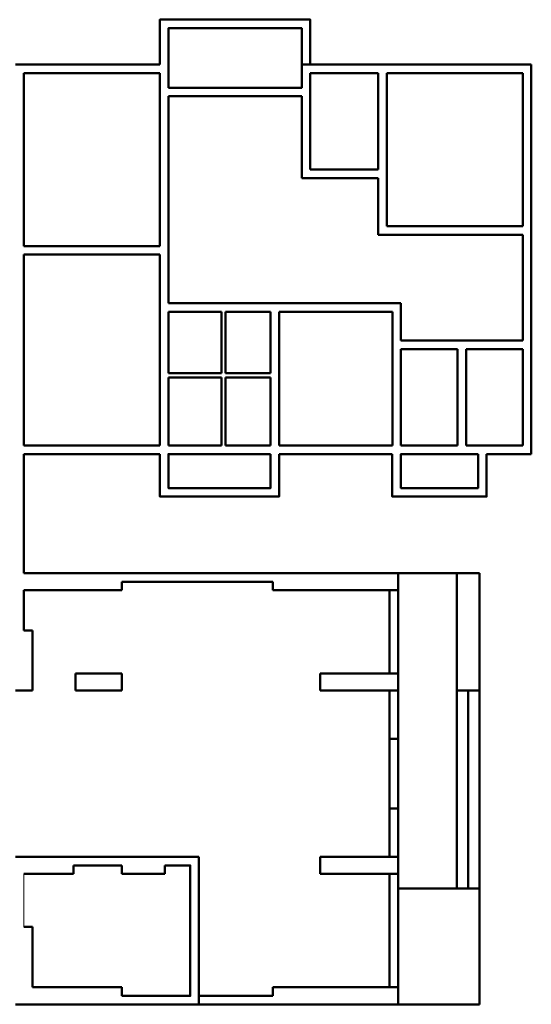
# Model space of a CAD drawing. Units: inches. Extents: x -105 to 1531, y -656 to 2003.
# Tile 6 of 6: x 979 to 1521, y 44 to 1085. Entities that reach past the tile are written whole.
import ezdxf

# ---------------------------------------------------------------- set-up
doc = ezdxf.new("R2010")
doc.units = ezdxf.units.IN
doc.header["$MEASUREMENT"] = 0
doc.layers.add('A-GLAZ', color=4, linetype='Continuous', lineweight=18)
doc.layers.add('A-WALL', color=7, linetype='Continuous', lineweight=50)

msp = doc.modelspace()

# ---------------------------------------------------------------- linework, layer by layer
at = {"layer": 'A-GLAZ'}
msp.add_line((984, 181.9), (984, 126), dxfattribs=at)
msp.add_line((984, 181.9), (984, 126), dxfattribs=at)
msp.add_line((984, 181.9), (984, 126), dxfattribs=at)
at = {"layer": 'A-WALL'}
for p, q in [((1278, 1076.5), (1137, 1076.5)), ((1278, 1013.5), (1278, 1076.5)), ((1128, 1038), (975, 1038)), ((1137, 1038), (1137, 1013.5)), ((1359, 1038), (1278, 1038)), ((1278, 1013.5), (1278, 1038)), ((1359, 1038), (1521, 1038)), ((1521, 737), (1521, 1038)), ((1128, 1029), (984, 1029)), ((984, 846), (984, 1029)), ((1128, 846), (1128, 1029)), ((1359, 1029), (1287, 1029)), ((1287, 927), (1287, 1029)), ((1359, 927), (1359, 1029)), ((1368, 1029), (1512, 1029)), ((1368, 867), (1368, 1029)), ((1512, 867), (1512, 1029)), ((1137, 1013.5), (1278, 1013.5)), ((1137, 1004.5), (1278, 1004.5)), ((1137, 1004.5), (1137, 837)), ((1278, 918), (1278, 1004.5)), ((1359, 927), (1287, 927)), ((1359, 918), (1278, 918)), ((1359, 858), (1359, 918)), ((1368, 867), (1512, 867)), ((1359, 858), (1512, 858)), ((1512, 746), (1512, 858)), ((984, 846), (1128, 846)), ((1137, 785.5), (1137, 846)), ((984, 635), (984, 837)), ((984, 837), (1128, 837)), ((1128, 635), (1128, 837)), ((1137, 785.5), (1383, 785.5)), ((1383, 746), (1383, 785.5)), ((1137, 776.5), (1193, 776.5)), ((1137, 711.5), (1137, 776.5)), ((1193, 711.5), (1193, 776.5)), ((1197.5, 776.5), (1245, 776.5)), ((1197.5, 711.5), (1197.5, 776.5)), ((1245, 711.5), (1245, 776.5)), ((1254, 635), (1254, 776.5)), ((1254, 776.5), (1374, 776.5)), ((1374, 635), (1374, 776.5)), ((984, 743.6), (984, 635)), ((1383, 746), (1512, 746)), ((1521, 626), (1521, 746)), ((1383, 635), (1383, 737)), ((1383, 737), (1443, 737)), ((1443, 635), (1443, 737)), ((1452, 635), (1452, 737)), ((1452, 737), (1512, 737)), ((1512, 635), (1512, 737)), ((1137, 711.5), (1193, 711.5)), ((1197.5, 711.5), (1245, 711.5)), ((1137, 635), (1137, 707)), ((1137, 707), (1193, 707)), ((1193, 635), (1193, 707)), ((1197.5, 635), (1197.5, 707)), ((1197.5, 707), (1245, 707)), ((1245, 635), (1245, 707)), ((984, 635), (1128, 635)), ((984, 626), (1128, 626)), ((984, 626), (984, 499.9)), ((1137, 635), (1193, 635)), ((1137, 626), (1137, 590)), ((1137, 626), (1245, 626)), ((1197.5, 635), (1245, 635)), ((1254, 635), (1374, 635)), ((1254, 626), (1373.9, 626)), ((1382.9, 626), (1382.9, 590)), ((1382.9, 626), (1464.7, 626)), ((1383, 635), (1443, 635)), ((1452, 635), (1512, 635)), ((1473.7, 626), (1521, 626)), ((984, 499.9), (1380, 499.9)), ((1380, 499.9), (1380, 43.9)), ((1442, 499.9), (1380, 499.9)), ((1442, 166.6), (1442, 499.9)), ((1442, 166.6), (1442, 499.9)), ((1442, 499.9), (1466, 499.9)), ((1466, 499.9), (1466, 166.6)), ((1087.6, 490.9), (1247.4, 490.9)), ((1087.6, 481.9), (1087.6, 490.9)), ((1247.4, 481.9), (1247.4, 490.9)), ((984, 481.9), (1087.6, 481.9)), ((984, 481.9), (984, 439.4)), ((1247.4, 481.9), (1380, 481.9)), ((1371, 481.9), (1371, 394)), ((984, 439.4), (993, 439.4)), ((993, 439.4), (993, 376)), ((1038.4, 376), (1038.4, 394)), ((1087.6, 394), (1038.4, 394)), ((1087.6, 376), (1087.6, 394)), ((1380, 394), (1297.6, 394)), ((1297.6, 376), (1297.6, 394)), ((984, 376), (975, 376)), ((993, 376), (984, 376)), ((1087.6, 376), (1038.4, 376)), ((1380, 376), (1297.6, 376)), ((1371, 324.9), (1371, 376)), ((1371, 376), (1371, 199.9)), ((1442, 376), (1466, 376)), ((1454, 376), (1454, 166.6)), ((1371, 324.9), (1380, 324.9)), ((1371, 250.9), (1371, 324.9)), ((1380, 324.9), (1380, 252.9)), ((1380, 250.9), (1371, 250.9)), ((1380, 252.9), (1380, 250.9)), ((1169, 199.9), (975, 199.9)), ((1169, 43.9), (1169, 199.9)), ((1297.6, 181.9), (1297.6, 199.9)), ((1297.6, 199.9), (1380, 199.9)), ((1036.5, 181.9), (1036.5, 190.9)), ((1087.6, 181.9), (1087.6, 190.9)), ((1133, 181.9), (1133, 190.9)), ((1297.6, 181.9), (1380, 181.9)), ((1371, 181.9), (1371, 61.9)), ((1466, 166.6), (1380, 166.6)), ((1466, 166.6), (1442, 166.6)), ((1466, 43.9), (1466, 166.6)), ((993, 126), (984, 126)), ((993, 61.9), (993, 126)), ((1087.6, 61.9), (993, 61.9)), ((1087.6, 52.9), (1087.6, 61.9)), ((1160, 52.9), (1087.6, 52.9)), ((1247.4, 52.9), (1169, 52.9)), ((1380, 61.9), (1247.4, 61.9)), ((1247.4, 52.9), (1247.4, 61.9)), ((975, 43.9), (984, 43.9)), ((1380, 43.9), (984, 43.9)), ((984, 43.9), (1169, 43.9)), ((1380, 43.9), (1440, 43.9)), ((1440, 43.9), (1442, 43.9)), ((1442, 43.9), (1454, 43.9)), ((1454, 43.9), (1466, 43.9))]:
    msp.add_line(p, q, dxfattribs=at)
for points in [[(1287, 1038), (1287, 1085.5), (1128, 1085.5), (1128, 1038)], [(1128, 1029), (1128, 1004.5)], [(1287, 1004.5), (1287, 1029)], [(1137, 1004.5), (1278, 1004.5)], [(984, 846), (984, 928.6)], [(984, 743.6), (984, 837)], [(1128, 626), (1128, 581), (1254, 581), (1254, 626)], [(1193, 635), (1137, 635)], [(1245, 635), (1197.5, 635)], [(1374, 635), (1373.9, 635)], [(1373.9, 626), (1373.9, 581), (1473.7, 581), (1473.7, 626)], [(1443, 635), (1383, 635)], [(1473.7, 635), (1473.7, 635), (1452, 635)], [(1087.6, 190.9), (1036.5, 190.9)], [(1087.6, 52.9), (1160, 52.9), (1160, 190.9), (1133, 190.9)], [(1036.5, 181.9), (984, 181.9)], [(1133, 181.9), (1087.6, 181.9)], [(1002, 61.9), (1087.6, 61.9)]]:
    msp.add_lwpolyline(points, dxfattribs=at)
for points in [[(1137, 1013.5), (1278, 1013.5), (1278, 1076.5), (1137, 1076.5)], [(1245, 626), (1137, 626), (1137, 590), (1245, 590)], [(1464.7, 626), (1382.9, 626), (1382.9, 590), (1464.7, 590)]]:
    msp.add_lwpolyline(points, close=True, dxfattribs=at)

doc.saveas('drawing.dxf')
